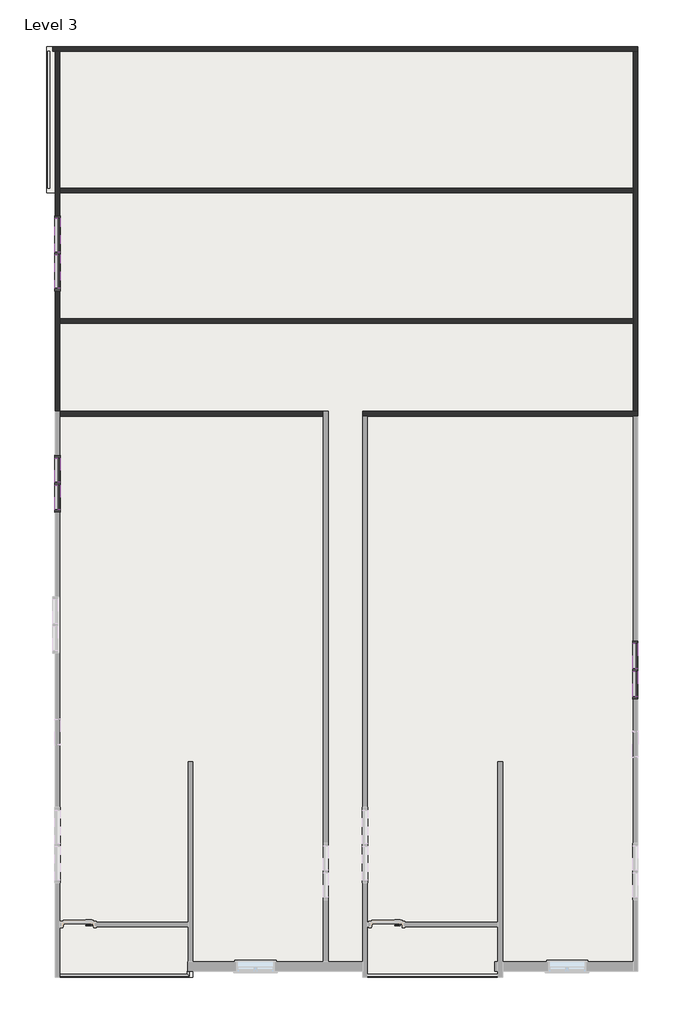
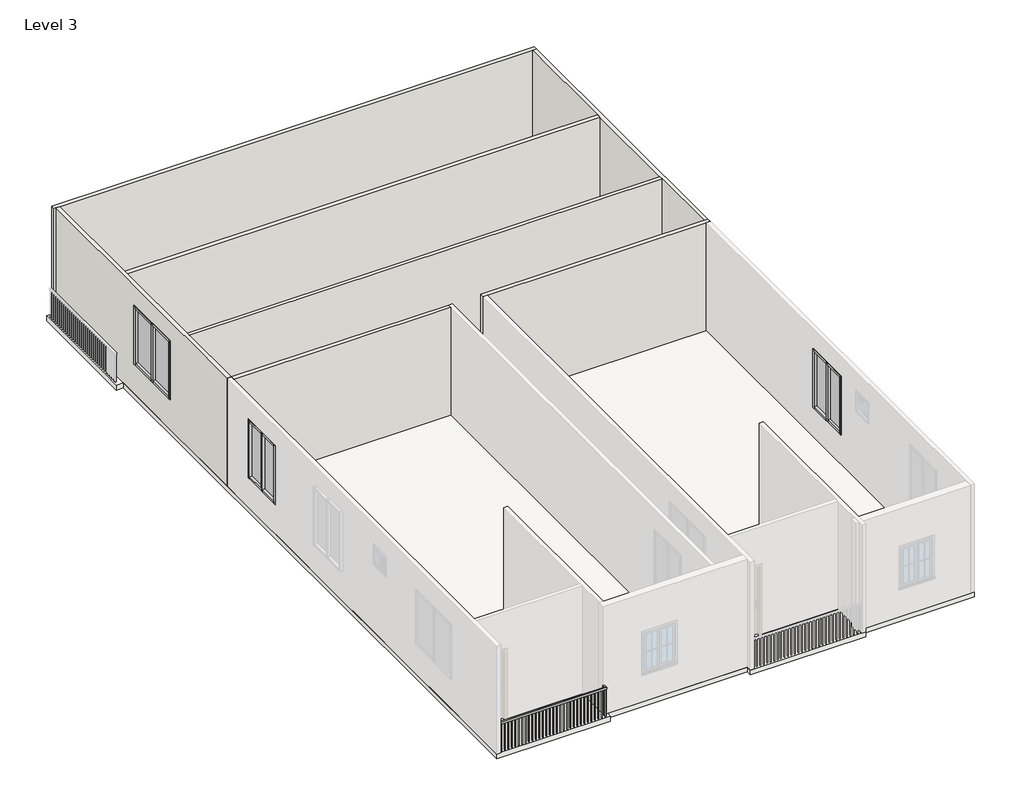
# One storey, part 2 of 3: 21 members, 7 walls, 6 plates, 1 railing, 1 slab.
"""IFC4 building model written with IfcOpenShell, lengths in millimetres."""

from ifc_helpers import new_model, si_unit, frame, origin, place, context, project, spatial, polyline, outline, extrude, faceted_brep, transform, mapped, element, save
from components import member_3f0e0172, member_96ae0c19, member_d60e8053, member_2fae0574, member_3e1d4a65, system_panel_glazed_c4393626, system_panel_glazed_d2c73f4b, system_panel_glazed_30879ba3

model = new_model("IFC4")

# Units and contexts
model_context = context("Model", 3, world=origin())
ifc_project = project(units=[si_unit("LENGTHUNIT", "METRE", prefix="MILLI")], contexts=[model_context])

# Site, building, storey
site = spatial("IfcSite", under=ifc_project)
building = spatial("IfcBuilding", under=site)
storey = spatial("IfcBuildingStorey", under=building, Name="Level 3", Elevation=6705.6)

# Members
placement = place(None, origin())
member_shape = member_3f0e0172(model_context)
element("IfcMember", 1, ObjectType="Rectangular Mullion : 2.5\" x 5\" rectangular", at=placement, inside=storey, context=model_context, shape_type="MappedRepresentation", body=[
    mapped(member_shape, transform((5848.1708786, -3933.7021821, 9448.8), x_axis=(0.0, 0.0, 1.0), y_axis=(-1.0, 0.0, 0.0), z_axis=(0.0, -1.0, 0.0))),
])
element("IfcMember", 2, ObjectType="Rectangular Mullion : 2.5\" x 5\" rectangular", at=placement, inside=storey, context=model_context, shape_type="MappedRepresentation", body=[
    mapped(member_shape, transform((5848.1708786, -3254.2521821, 9448.8), x_axis=(0.0, 0.0, 1.0), y_axis=(-1.0, 0.0, 0.0), z_axis=(0.0, -1.0, 0.0))),
])
element("IfcMember", 3, ObjectType="Rectangular Mullion : 2.5\" x 5\" rectangular", at=placement, inside=storey, context=model_context, shape_type="MappedRepresentation", body=[
    mapped(member_shape, transform((5848.1708786, -2638.3021821, 7620.0), x_axis=(0.0, 0.0, -1.0), y_axis=(-1.0, 0.0, 0.0), z_axis=(0.0, 1.0, 0.0))),
])
element("IfcMember", 4, ObjectType="Rectangular Mullion : 2.5\" x 5\" rectangular", at=placement, inside=storey, context=model_context, shape_type="MappedRepresentation", body=[
    mapped(member_shape, transform((5848.1708786, -3317.7521821, 7620.0), x_axis=(0.0, 0.0, -1.0), y_axis=(-1.0, 0.0, 0.0), z_axis=(0.0, 1.0, 0.0))),
])
member_2_shape = member_96ae0c19(model_context)
element("IfcMember", 5, ObjectType="Rectangular Mullion : 2.5\" x 5\" rectangular", at=placement, inside=storey, context=model_context, shape_type="MappedRepresentation", body=[
    mapped(member_2_shape, transform((-8153.157583, 600.1666267, 9448.8), x_axis=(0.0, 0.0, 1.0), y_axis=(-1.0, 0.0, 0.0), z_axis=(0.0, -1.0, 0.0))),
])
element("IfcMember", 6, ObjectType="Rectangular Mullion : 2.5\" x 5\" rectangular", at=placement, inside=storey, context=model_context, shape_type="MappedRepresentation", body=[
    mapped(member_2_shape, transform((-8153.157583, 1254.9937905, 9448.8), x_axis=(0.0, 0.0, 1.0), y_axis=(-1.0, 0.0, 0.0), z_axis=(0.0, -1.0, 0.0))),
])
element("IfcMember", 7, ObjectType="Rectangular Mullion : 2.5\" x 5\" rectangular", at=placement, inside=storey, context=model_context, shape_type="MappedRepresentation", body=[
    mapped(member_2_shape, transform((-8153.157583, 1846.3209543, 7620.0), x_axis=(0.0, 0.0, -1.0), y_axis=(-1.0, 0.0, 0.0), z_axis=(0.0, 1.0, 0.0))),
])
element("IfcMember", 8, ObjectType="Rectangular Mullion : 2.5\" x 5\" rectangular", at=placement, inside=storey, context=model_context, shape_type="MappedRepresentation", body=[
    mapped(member_2_shape, transform((-8153.157583, 1191.4937905, 7620.0), x_axis=(0.0, 0.0, -1.0), y_axis=(-1.0, 0.0, 0.0), z_axis=(0.0, 1.0, 0.0))),
])
member_3_shape = member_d60e8053(model_context)
element("IfcMember", 9, ObjectType="Rectangular Mullion : 2.5\" x 5\" rectangular", at=placement, inside=storey, context=model_context, shape_type="MappedRepresentation", body=[
    mapped(member_3_shape, transform((5848.1708786, -3286.0021821, 7620.0), x_axis=(0.0, -1.0, 0.0), y_axis=(-1.0, 0.0, 0.0), z_axis=(0.0, 0.0, -1.0))),
])
element("IfcMember", 10, ObjectType="Rectangular Mullion : 2.5\" x 5\" rectangular", at=placement, inside=storey, context=model_context, shape_type="MappedRepresentation", body=[
    mapped(member_3_shape, transform((-8153.157583, 1223.2437905, 7620.0), x_axis=(0.0, -1.0, 0.0), y_axis=(-1.0, 0.0, 0.0), z_axis=(0.0, 0.0, -1.0))),
])
element("IfcMember", 11, ObjectType="Rectangular Mullion : 2.5\" x 5\" rectangular", at=placement, inside=storey, context=model_context, shape_type="MappedRepresentation", body=[
    mapped(member_3_shape, transform((-8153.157583, 6807.1511393, 7620.0), x_axis=(0.0, -1.0, 0.0), y_axis=(-1.0, 0.0, 0.0), z_axis=(0.0, 0.0, -1.0))),
])
member_4_shape = member_2fae0574(model_context)
element("IfcMember", 12, ObjectType="Rectangular Mullion : 2.5\" x 5\" rectangular", at=placement, inside=storey, context=model_context, shape_type="MappedRepresentation", body=[
    mapped(member_4_shape, transform((5848.1708786, -2574.8021821, 9448.8), x_axis=(0.0, 1.0, 0.0), y_axis=(-1.0, 0.0, 0.0), z_axis=(0.0, 0.0, 1.0))),
])
element("IfcMember", 13, ObjectType="Rectangular Mullion : 2.5\" x 5\" rectangular", at=placement, inside=storey, context=model_context, shape_type="MappedRepresentation", body=[
    mapped(member_4_shape, transform((-8153.157583, 1909.8209543, 9448.8), x_axis=(0.0, 1.0, 0.0), y_axis=(-1.0, 0.0, 0.0), z_axis=(0.0, 0.0, 1.0))),
])
element("IfcMember", 14, ObjectType="Rectangular Mullion : 2.5\" x 5\" rectangular", at=placement, inside=storey, context=model_context, shape_type="MappedRepresentation", body=[
    mapped(member_4_shape, transform((-8153.157583, 7721.9533991, 9448.8), x_axis=(0.0, 1.0, 0.0), y_axis=(-1.0, 0.0, 0.0), z_axis=(0.0, 0.0, 1.0))),
])
element("IfcMember", 15, ObjectType="Rectangular Mullion : 2.5\" x 5\" rectangular", at=placement, inside=storey, context=model_context, shape_type="MappedRepresentation", body=[
    mapped(member_4_shape, transform((5848.1708786, -3997.2021821, 7620.0), x_axis=(0.0, -1.0, 0.0), y_axis=(-1.0, 0.0, 0.0), z_axis=(0.0, 0.0, -1.0))),
])
element("IfcMember", 16, ObjectType="Rectangular Mullion : 2.5\" x 5\" rectangular", at=placement, inside=storey, context=model_context, shape_type="MappedRepresentation", body=[
    mapped(member_4_shape, transform((-8153.157583, 536.6666267, 7620.0), x_axis=(0.0, -1.0, 0.0), y_axis=(-1.0, 0.0, 0.0), z_axis=(0.0, 0.0, -1.0))),
])
element("IfcMember", 17, ObjectType="Rectangular Mullion : 2.5\" x 5\" rectangular", at=placement, inside=storey, context=model_context, shape_type="MappedRepresentation", body=[
    mapped(member_4_shape, transform((-8153.157583, 5892.3488795, 7620.0), x_axis=(0.0, -1.0, 0.0), y_axis=(-1.0, 0.0, 0.0), z_axis=(0.0, 0.0, -1.0))),
])
member_5_shape = member_3e1d4a65(model_context)
element("IfcMember", 18, ObjectType="Rectangular Mullion : 2.5\" x 5\" rectangular", at=placement, inside=storey, context=model_context, shape_type="MappedRepresentation", body=[
    mapped(member_5_shape, transform((-8153.157583, 5955.8488795, 9448.8), x_axis=(0.0, 0.0, 1.0), y_axis=(-1.0, 0.0, 0.0), z_axis=(0.0, -1.0, 0.0))),
])
element("IfcMember", 19, ObjectType="Rectangular Mullion : 2.5\" x 5\" rectangular", at=placement, inside=storey, context=model_context, shape_type="MappedRepresentation", body=[
    mapped(member_5_shape, transform((-8153.157583, 6838.9011393, 9448.8), x_axis=(0.0, 0.0, 1.0), y_axis=(-1.0, 0.0, 0.0), z_axis=(0.0, -1.0, 0.0))),
])
element("IfcMember", 20, ObjectType="Rectangular Mullion : 2.5\" x 5\" rectangular", at=placement, inside=storey, context=model_context, shape_type="MappedRepresentation", body=[
    mapped(member_5_shape, transform((-8153.157583, 7658.4533991, 7620.0), x_axis=(0.0, 0.0, -1.0), y_axis=(-1.0, 0.0, 0.0), z_axis=(0.0, 1.0, 0.0))),
])
element("IfcMember", 21, ObjectType="Rectangular Mullion : 2.5\" x 5\" rectangular", at=placement, inside=storey, context=model_context, shape_type="MappedRepresentation", body=[
    mapped(member_5_shape, transform((-8153.157583, 6775.4011393, 7620.0), x_axis=(0.0, 0.0, -1.0), y_axis=(-1.0, 0.0, 0.0), z_axis=(0.0, 1.0, 0.0))),
])

# Plates
system_panel_glazed_shape = system_panel_glazed_c4393626(model_context)
element("IfcPlate", 22, ObjectType="System Panel : Glazed", at=placement, inside=storey, context=model_context, shape_type="MappedRepresentation", body=[
    mapped(system_panel_glazed_shape, transform((-8153.157583, 1550.6573724, 7683.5), x_axis=(0.0, -1.0, 0.0), y_axis=(1.0, 0.0, 0.0), z_axis=(0.0, 0.0, 1.0))),
])
element("IfcPlate", 23, ObjectType="System Panel : Glazed", at=placement, inside=storey, context=model_context, shape_type="MappedRepresentation", body=[
    mapped(system_panel_glazed_shape, transform((-8153.157583, 895.8302086, 7683.5), x_axis=(0.0, -1.0, 0.0), y_axis=(1.0, 0.0, 0.0), z_axis=(0.0, 0.0, 1.0))),
])
system_panel_glazed_2_shape = system_panel_glazed_d2c73f4b(model_context)
element("IfcPlate", 24, ObjectType="System Panel : Glazed", at=placement, inside=storey, context=model_context, shape_type="MappedRepresentation", body=[
    mapped(system_panel_glazed_2_shape, transform((5848.1708786, -2946.2771821, 7683.5), x_axis=(0.0, -1.0, 0.0), y_axis=(1.0, 0.0, 0.0), z_axis=(0.0, 0.0, 1.0))),
])
element("IfcPlate", 25, ObjectType="System Panel : Glazed", at=placement, inside=storey, context=model_context, shape_type="MappedRepresentation", body=[
    mapped(system_panel_glazed_2_shape, transform((5848.1708786, -3625.7271821, 7683.5), x_axis=(0.0, -1.0, 0.0), y_axis=(1.0, 0.0, 0.0), z_axis=(0.0, 0.0, 1.0))),
])
system_panel_glazed_3_shape = system_panel_glazed_30879ba3(model_context)
element("IfcPlate", 26, ObjectType="System Panel : Glazed", at=placement, inside=storey, context=model_context, shape_type="MappedRepresentation", body=[
    mapped(system_panel_glazed_3_shape, transform((-8153.157583, 7248.6772692, 7683.5), x_axis=(0.0, -1.0, 0.0), y_axis=(1.0, 0.0, 0.0), z_axis=(0.0, 0.0, 1.0))),
])
element("IfcPlate", 27, ObjectType="System Panel : Glazed", at=placement, inside=storey, context=model_context, shape_type="MappedRepresentation", body=[
    mapped(system_panel_glazed_3_shape, transform((-8153.157583, 6365.6250094, 7683.5), x_axis=(0.0, -1.0, 0.0), y_axis=(1.0, 0.0, 0.0), z_axis=(0.0, 0.0, 1.0))),
])

# Railing
element("IfcRailing", 28, ObjectType="Handrail - Rectangular", at=placement, inside=storey, context=model_context, shape_type="SolidModel", body=[
    faceted_brep([(-8153.157583, -10659.0005933, 7620.0), (-8153.157583, -10659.0005933, 7569.2), (-8153.157583, -10709.8005933, 7569.2), (-8153.157583, -10709.8005933, 7620.0), (-5014.0237038, -10659.0005933, 7620.0), (-5014.0237038, -10659.0005933, 7569.2), (-4963.2237038, -10709.8005933, 7569.2), (-4963.2237038, -10709.8005933, 7620.0), (-5014.0237038, -10582.0742041, 7620.0), (-4963.2237038, -10582.0742041, 7620.0), (-4963.2237038, -10582.0742041, 7569.2), (-5014.0237038, -10582.0742041, 7569.2)], [[[0, 1, 2, 3]], [[1, 0, 4, 5]], [[2, 1, 5, 6]], [[3, 2, 6, 7]], [[0, 3, 7, 4]], [[8, 9, 10, 11]], [[5, 4, 8, 11]], [[6, 5, 11, 10]], [[7, 6, 10, 9]], [[4, 7, 9, 8]]]),
    extrude(outline(polyline([(-4979.0987038, -10592.3255933), (-4998.1487038, -10592.3255933), (-4998.1487038, -10573.2755933), (-4979.0987038, -10573.2755933), (-4979.0987038, -10592.3255933)])), frame((0.0, 0.0, 6705.6), z_axis=(0.0, 0.0, 1.0), x_axis=(1.0, 0.0, 0.0)), (0.0, 0.0, 1.0), 863.6),
    extrude(outline(polyline([(-5013.082583, -10693.9255933), (-5013.082583, -10674.8755933), (-4994.032583, -10674.8755933), (-4994.032583, -10693.9255933), (-5013.082583, -10693.9255933)])), frame((0.0, 0.0, 6705.6), z_axis=(0.0, 0.0, 1.0), x_axis=(1.0, 0.0, 0.0)), (0.0, 0.0, 1.0), 863.6),
    extrude(outline(polyline([(-5114.682583, -10693.9255933), (-5114.682583, -10674.8755933), (-5095.632583, -10674.8755933), (-5095.632583, -10693.9255933), (-5114.682583, -10693.9255933)])), frame((0.0, 0.0, 6705.6), z_axis=(0.0, 0.0, 1.0), x_axis=(1.0, 0.0, 0.0)), (0.0, 0.0, 1.0), 863.6),
    extrude(outline(polyline([(-5216.282583, -10693.9255933), (-5216.282583, -10674.8755933), (-5197.232583, -10674.8755933), (-5197.232583, -10693.9255933), (-5216.282583, -10693.9255933)])), frame((0.0, 0.0, 6705.6), z_axis=(0.0, 0.0, 1.0), x_axis=(1.0, 0.0, 0.0)), (0.0, 0.0, 1.0), 863.6),
    extrude(outline(polyline([(-5317.882583, -10693.9255933), (-5317.882583, -10674.8755933), (-5298.832583, -10674.8755933), (-5298.832583, -10693.9255933), (-5317.882583, -10693.9255933)])), frame((0.0, 0.0, 6705.6), z_axis=(0.0, 0.0, 1.0), x_axis=(1.0, 0.0, 0.0)), (0.0, 0.0, 1.0), 863.6),
    extrude(outline(polyline([(-5419.482583, -10693.9255933), (-5419.482583, -10674.8755933), (-5400.432583, -10674.8755933), (-5400.432583, -10693.9255933), (-5419.482583, -10693.9255933)])), frame((0.0, 0.0, 6705.6), z_axis=(0.0, 0.0, 1.0), x_axis=(1.0, 0.0, 0.0)), (0.0, 0.0, 1.0), 863.6),
    extrude(outline(polyline([(-5521.082583, -10693.9255933), (-5521.082583, -10674.8755933), (-5502.032583, -10674.8755933), (-5502.032583, -10693.9255933), (-5521.082583, -10693.9255933)])), frame((0.0, 0.0, 6705.6), z_axis=(0.0, 0.0, 1.0), x_axis=(1.0, 0.0, 0.0)), (0.0, 0.0, 1.0), 863.6),
    extrude(outline(polyline([(-5622.682583, -10693.9255933), (-5622.682583, -10674.8755933), (-5603.632583, -10674.8755933), (-5603.632583, -10693.9255933), (-5622.682583, -10693.9255933)])), frame((0.0, 0.0, 6705.6), z_axis=(0.0, 0.0, 1.0), x_axis=(1.0, 0.0, 0.0)), (0.0, 0.0, 1.0), 863.6),
    extrude(outline(polyline([(-5724.282583, -10693.9255933), (-5724.282583, -10674.8755933), (-5705.232583, -10674.8755933), (-5705.232583, -10693.9255933), (-5724.282583, -10693.9255933)])), frame((0.0, 0.0, 6705.6), z_axis=(0.0, 0.0, 1.0), x_axis=(1.0, 0.0, 0.0)), (0.0, 0.0, 1.0), 863.6),
    extrude(outline(polyline([(-5825.882583, -10693.9255933), (-5825.882583, -10674.8755933), (-5806.832583, -10674.8755933), (-5806.832583, -10693.9255933), (-5825.882583, -10693.9255933)])), frame((0.0, 0.0, 6705.6), z_axis=(0.0, 0.0, 1.0), x_axis=(1.0, 0.0, 0.0)), (0.0, 0.0, 1.0), 863.6),
    extrude(outline(polyline([(-5927.482583, -10693.9255933), (-5927.482583, -10674.8755933), (-5908.432583, -10674.8755933), (-5908.432583, -10693.9255933), (-5927.482583, -10693.9255933)])), frame((0.0, 0.0, 6705.6), z_axis=(0.0, 0.0, 1.0), x_axis=(1.0, 0.0, 0.0)), (0.0, 0.0, 1.0), 863.6),
    extrude(outline(polyline([(-6029.082583, -10693.9255933), (-6029.082583, -10674.8755933), (-6010.032583, -10674.8755933), (-6010.032583, -10693.9255933), (-6029.082583, -10693.9255933)])), frame((0.0, 0.0, 6705.6), z_axis=(0.0, 0.0, 1.0), x_axis=(1.0, 0.0, 0.0)), (0.0, 0.0, 1.0), 863.6),
    extrude(outline(polyline([(-6130.682583, -10693.9255933), (-6130.682583, -10674.8755933), (-6111.632583, -10674.8755933), (-6111.632583, -10693.9255933), (-6130.682583, -10693.9255933)])), frame((0.0, 0.0, 6705.6), z_axis=(0.0, 0.0, 1.0), x_axis=(1.0, 0.0, 0.0)), (0.0, 0.0, 1.0), 863.6),
    extrude(outline(polyline([(-6232.282583, -10693.9255933), (-6232.282583, -10674.8755933), (-6213.232583, -10674.8755933), (-6213.232583, -10693.9255933), (-6232.282583, -10693.9255933)])), frame((0.0, 0.0, 6705.6), z_axis=(0.0, 0.0, 1.0), x_axis=(1.0, 0.0, 0.0)), (0.0, 0.0, 1.0), 863.6),
    extrude(outline(polyline([(-6333.882583, -10693.9255933), (-6333.882583, -10674.8755933), (-6314.832583, -10674.8755933), (-6314.832583, -10693.9255933), (-6333.882583, -10693.9255933)])), frame((0.0, 0.0, 6705.6), z_axis=(0.0, 0.0, 1.0), x_axis=(1.0, 0.0, 0.0)), (0.0, 0.0, 1.0), 863.6),
    extrude(outline(polyline([(-6435.482583, -10693.9255933), (-6435.482583, -10674.8755933), (-6416.432583, -10674.8755933), (-6416.432583, -10693.9255933), (-6435.482583, -10693.9255933)])), frame((0.0, 0.0, 6705.6), z_axis=(0.0, 0.0, 1.0), x_axis=(1.0, 0.0, 0.0)), (0.0, 0.0, 1.0), 863.6),
    extrude(outline(polyline([(-6537.082583, -10693.9255933), (-6537.082583, -10674.8755933), (-6518.032583, -10674.8755933), (-6518.032583, -10693.9255933), (-6537.082583, -10693.9255933)])), frame((0.0, 0.0, 6705.6), z_axis=(0.0, 0.0, 1.0), x_axis=(1.0, 0.0, 0.0)), (0.0, 0.0, 1.0), 863.6),
    extrude(outline(polyline([(-6638.682583, -10693.9255933), (-6638.682583, -10674.8755933), (-6619.632583, -10674.8755933), (-6619.632583, -10693.9255933), (-6638.682583, -10693.9255933)])), frame((0.0, 0.0, 6705.6), z_axis=(0.0, 0.0, 1.0), x_axis=(1.0, 0.0, 0.0)), (0.0, 0.0, 1.0), 863.6),
    extrude(outline(polyline([(-6740.282583, -10693.9255933), (-6740.282583, -10674.8755933), (-6721.232583, -10674.8755933), (-6721.232583, -10693.9255933), (-6740.282583, -10693.9255933)])), frame((0.0, 0.0, 6705.6), z_axis=(0.0, 0.0, 1.0), x_axis=(1.0, 0.0, 0.0)), (0.0, 0.0, 1.0), 863.6),
    extrude(outline(polyline([(-6841.882583, -10693.9255933), (-6841.882583, -10674.8755933), (-6822.832583, -10674.8755933), (-6822.832583, -10693.9255933), (-6841.882583, -10693.9255933)])), frame((0.0, 0.0, 6705.6), z_axis=(0.0, 0.0, 1.0), x_axis=(1.0, 0.0, 0.0)), (0.0, 0.0, 1.0), 863.6),
    extrude(outline(polyline([(-6943.482583, -10693.9255933), (-6943.482583, -10674.8755933), (-6924.432583, -10674.8755933), (-6924.432583, -10693.9255933), (-6943.482583, -10693.9255933)])), frame((0.0, 0.0, 6705.6), z_axis=(0.0, 0.0, 1.0), x_axis=(1.0, 0.0, 0.0)), (0.0, 0.0, 1.0), 863.6),
    extrude(outline(polyline([(-7045.082583, -10693.9255933), (-7045.082583, -10674.8755933), (-7026.032583, -10674.8755933), (-7026.032583, -10693.9255933), (-7045.082583, -10693.9255933)])), frame((0.0, 0.0, 6705.6), z_axis=(0.0, 0.0, 1.0), x_axis=(1.0, 0.0, 0.0)), (0.0, 0.0, 1.0), 863.6),
    extrude(outline(polyline([(-7146.682583, -10693.9255933), (-7146.682583, -10674.8755933), (-7127.632583, -10674.8755933), (-7127.632583, -10693.9255933), (-7146.682583, -10693.9255933)])), frame((0.0, 0.0, 6705.6), z_axis=(0.0, 0.0, 1.0), x_axis=(1.0, 0.0, 0.0)), (0.0, 0.0, 1.0), 863.6),
    extrude(outline(polyline([(-7248.282583, -10693.9255933), (-7248.282583, -10674.8755933), (-7229.232583, -10674.8755933), (-7229.232583, -10693.9255933), (-7248.282583, -10693.9255933)])), frame((0.0, 0.0, 6705.6), z_axis=(0.0, 0.0, 1.0), x_axis=(1.0, 0.0, 0.0)), (0.0, 0.0, 1.0), 863.6),
    extrude(outline(polyline([(-7349.882583, -10693.9255933), (-7349.882583, -10674.8755933), (-7330.832583, -10674.8755933), (-7330.832583, -10693.9255933), (-7349.882583, -10693.9255933)])), frame((0.0, 0.0, 6705.6), z_axis=(0.0, 0.0, 1.0), x_axis=(1.0, 0.0, 0.0)), (0.0, 0.0, 1.0), 863.6),
    extrude(outline(polyline([(-7451.482583, -10693.9255933), (-7451.482583, -10674.8755933), (-7432.432583, -10674.8755933), (-7432.432583, -10693.9255933), (-7451.482583, -10693.9255933)])), frame((0.0, 0.0, 6705.6), z_axis=(0.0, 0.0, 1.0), x_axis=(1.0, 0.0, 0.0)), (0.0, 0.0, 1.0), 863.6),
    extrude(outline(polyline([(-7553.082583, -10693.9255933), (-7553.082583, -10674.8755933), (-7534.032583, -10674.8755933), (-7534.032583, -10693.9255933), (-7553.082583, -10693.9255933)])), frame((0.0, 0.0, 6705.6), z_axis=(0.0, 0.0, 1.0), x_axis=(1.0, 0.0, 0.0)), (0.0, 0.0, 1.0), 863.6),
    extrude(outline(polyline([(-7654.682583, -10693.9255933), (-7654.682583, -10674.8755933), (-7635.632583, -10674.8755933), (-7635.632583, -10693.9255933), (-7654.682583, -10693.9255933)])), frame((0.0, 0.0, 6705.6), z_axis=(0.0, 0.0, 1.0), x_axis=(1.0, 0.0, 0.0)), (0.0, 0.0, 1.0), 863.6),
    extrude(outline(polyline([(-7756.282583, -10693.9255933), (-7756.282583, -10674.8755933), (-7737.232583, -10674.8755933), (-7737.232583, -10693.9255933), (-7756.282583, -10693.9255933)])), frame((0.0, 0.0, 6705.6), z_axis=(0.0, 0.0, 1.0), x_axis=(1.0, 0.0, 0.0)), (0.0, 0.0, 1.0), 863.6),
    extrude(outline(polyline([(-7857.882583, -10693.9255933), (-7857.882583, -10674.8755933), (-7838.832583, -10674.8755933), (-7838.832583, -10693.9255933), (-7857.882583, -10693.9255933)])), frame((0.0, 0.0, 6705.6), z_axis=(0.0, 0.0, 1.0), x_axis=(1.0, 0.0, 0.0)), (0.0, 0.0, 1.0), 863.6),
    extrude(outline(polyline([(-7959.482583, -10693.9255933), (-7959.482583, -10674.8755933), (-7940.432583, -10674.8755933), (-7940.432583, -10693.9255933), (-7959.482583, -10693.9255933)])), frame((0.0, 0.0, 6705.6), z_axis=(0.0, 0.0, 1.0), x_axis=(1.0, 0.0, 0.0)), (0.0, 0.0, 1.0), 863.6),
    extrude(outline(polyline([(-8061.082583, -10693.9255933), (-8061.082583, -10674.8755933), (-8042.032583, -10674.8755933), (-8042.032583, -10693.9255933), (-8061.082583, -10693.9255933)])), frame((0.0, 0.0, 6705.6), z_axis=(0.0, 0.0, 1.0), x_axis=(1.0, 0.0, 0.0)), (0.0, 0.0, 1.0), 863.6),
    extrude(outline(polyline([(-4998.1487038, -10693.9255933), (-4998.1487038, -10674.8755933), (-4979.0987038, -10674.8755933), (-4979.0987038, -10693.9255933), (-4998.1487038, -10693.9255933)])), frame((0.0, 0.0, 6705.6), z_axis=(0.0, 0.0, 1.0), x_axis=(1.0, 0.0, 0.0)), (0.0, 0.0, 1.0), 863.6),
    extrude(outline(polyline([(-4979.0987038, -10601.1242041), (-4998.1487038, -10601.1242041), (-4998.1487038, -10582.0742041), (-4979.0987038, -10582.0742041), (-4979.0987038, -10601.1242041)])), frame((0.0, 0.0, 6705.6), z_axis=(0.0, 0.0, 1.0), x_axis=(1.0, 0.0, 0.0)), (0.0, 0.0, 1.0), 863.6),
    extrude(outline(polyline([(-8153.157583, -10693.9255933), (-8153.157583, -10674.8755933), (-8134.107583, -10674.8755933), (-8134.107583, -10693.9255933), (-8153.157583, -10693.9255933)])), frame((0.0, 0.0, 6705.6), z_axis=(0.0, 0.0, 1.0), x_axis=(1.0, 0.0, 0.0)), (0.0, 0.0, 1.0), 863.6),
])

# Slab
element("IfcSlab", 29, ObjectType="6\" floor", at=placement, inside=storey, context=model_context, shape_type="SweptSolid", body=[
    extrude(outline(polyline([(5905.3208786, 11818.2189683), (5905.3208786, -10585.8779557), (2630.290751, -10585.8779557), (2630.290751, -10737.6531157), (-762.8431282, -10737.6531157), (-762.8431282, -10585.8779557), (-4874.3237038, -10585.8779557), (-4874.3237038, -10733.8493641), (-8210.307583, -10733.8493641), (-8210.307583, 8277.3011327), (-8419.607647, 8277.3011327), (-8419.607647, 11818.2189683), (5905.3208786, 11818.2189683)])), frame((0.0, 0.0, 6553.2), z_axis=(0.0, 0.0, 1.0), x_axis=(1.0, 0.0, 0.0)), (0.0, 0.0, 1.0), 152.4),
])

# Walls
element("IfcWall", 30, ObjectType="4.5\" wall", at=placement, inside=storey, context=model_context, shape_type="Brep", body=[
    faceted_brep([(-8267.457583, 11703.9189683, 6705.6), (-8210.307583, 11703.9189683, 6705.6), (-8096.007583, 11703.9189683, 6705.6), (5791.0208786, 11703.9189683, 6705.6), (5905.3208786, 11703.9189683, 6705.6), (5905.3208786, 11703.9189683, 10058.4), (5791.0208786, 11703.9189683, 10058.4), (-8096.007583, 11703.9189683, 10058.4), (-8210.307583, 11703.9189683, 10058.4), (-8267.457583, 11703.9189683, 10058.4), (-8267.457583, 11818.2189683, 6705.6), (-8267.457583, 11818.2189683, 10058.4), (5905.3208786, 11818.2189683, 10058.4), (5905.3208786, 11818.2189683, 6705.6)], [[[0, 1, 2, 3, 4, 5, 6, 7, 8, 9]], [[10, 11, 12, 13]], [[4, 3, 2, 1, 0, 10, 13]], [[9, 8, 7, 6, 5, 12, 11]], [[0, 9, 11, 10]], [[5, 4, 13, 12]]]),
])
element("IfcWall", 31, ObjectType="4.5\" wall", at=placement, inside=storey, context=model_context, shape_type="Brep", body=[
    faceted_brep([(5791.0208786, 11703.9189683, 6705.6), (5791.0208786, 8387.4224771, 6705.6), (5791.0208786, 8273.1224771, 6705.6), (5791.0208786, 5226.5048975, 6705.6), (5791.0208786, 5112.2048975, 6705.6), (5791.0208786, 2978.3002499, 6705.6), (5791.0208786, 2978.3002499, 10058.4), (5791.0208786, 5112.2048975, 10058.4), (5791.0208786, 5226.5048975, 10058.4), (5791.0208786, 8273.1224771, 10058.4), (5791.0208786, 8387.4224771, 10058.4), (5791.0208786, 11703.9189683, 10058.4), (5905.3208786, 11703.9189683, 6705.6), (5905.3208786, 11703.9189683, 10058.4), (5905.3208786, 2978.3002499, 10058.4), (5905.3208786, 2978.3002499, 6705.6)], [[[0, 1, 2, 3, 4, 5, 6, 7, 8, 9, 10, 11]], [[12, 13, 14, 15]], [[5, 4, 3, 2, 1, 0, 12, 15]], [[11, 10, 9, 8, 7, 6, 14, 13]], [[0, 11, 13, 12]], [[6, 5, 15, 14]]]),
])
element("IfcWall", 32, ObjectType="4.5\" wall", at=placement, inside=storey, context=model_context, shape_type="SweptSolid", body=[
    extrude(outline(polyline([(-1713.5935762, 2864.0002499), (-8096.007583, 2864.0002499), (-8096.007583, 2978.3002499), (-1713.5935762, 2978.3002499), (-1713.5935762, 2864.0002499)])), frame((0.0, 0.0, 6705.6), z_axis=(0.0, 0.0, 1.0), x_axis=(1.0, 0.0, 0.0)), (0.0, 0.0, 1.0), 3352.8),
])
element("IfcWall", 33, ObjectType="4.5\" wall", at=placement, inside=storey, context=model_context, shape_type="SweptSolid", body=[
    extrude(outline(polyline([(-8096.007583, 5226.5048975), (5791.0208786, 5226.5048975), (5791.0208786, 5112.2048975), (-8096.007583, 5112.2048975), (-8096.007583, 5226.5048975)])), frame((0.0, 0.0, 6705.6), z_axis=(0.0, 0.0, 1.0), x_axis=(1.0, 0.0, 0.0)), (0.0, 0.0, 1.0), 3352.8),
])
element("IfcWall", 34, ObjectType="4.5\" wall", at=placement, inside=storey, context=model_context, shape_type="SweptSolid", body=[
    extrude(outline(polyline([(-8096.007583, 8387.4224771), (5791.0208786, 8387.4224771), (5791.0208786, 8273.1224771), (-8096.007583, 8273.1224771), (-8096.007583, 8387.4224771)])), frame((0.0, 0.0, 6705.6), z_axis=(0.0, 0.0, 1.0), x_axis=(1.0, 0.0, 0.0)), (0.0, 0.0, 1.0), 3352.8),
])
element("IfcWall", 35, ObjectType="4.5\" wall", at=placement, inside=storey, context=model_context, shape_type="Brep", body=[
    faceted_brep([(-8096.007583, 2978.3002499, 6705.6), (-8096.007583, 5112.2048975, 6705.6), (-8096.007583, 5226.5048975, 6705.6), (-8096.007583, 8273.1224771, 6705.6), (-8096.007583, 8387.4224771, 6705.6), (-8096.007583, 11703.9189683, 6705.6), (-8096.007583, 11703.9189683, 10058.4), (-8096.007583, 8387.4224771, 10058.4), (-8096.007583, 8273.1224771, 10058.4), (-8096.007583, 5226.5048975, 10058.4), (-8096.007583, 5112.2048975, 10058.4), (-8096.007583, 2978.3002499, 10058.4), (-8096.007583, 7721.9533991, 9448.8), (-8096.007583, 7721.9533991, 7620.0), (-8096.007583, 5892.3488795, 7620.0), (-8096.007583, 5892.3488795, 9448.8), (-8210.307583, 11703.9189683, 6705.6), (-8210.307583, 2978.3002499, 6705.6), (-8210.307583, 2978.3002499, 10058.4), (-8210.307583, 11703.9189683, 10058.4), (-8210.307583, 7721.9533991, 7620.0), (-8210.307583, 7721.9533991, 9448.8), (-8210.307583, 5892.3488795, 9448.8), (-8210.307583, 5892.3488795, 7620.0)], [[[0, 1, 2, 3, 4, 5, 6, 7, 8, 9, 10, 11], [12, 13, 14, 15]], [[16, 17, 18, 19], [20, 21, 22, 23]], [[5, 4, 3, 2, 1, 0, 17, 16]], [[11, 10, 9, 8, 7, 6, 19, 18]], [[6, 5, 16, 19]], [[0, 11, 18, 17]], [[20, 13, 12, 21]], [[21, 12, 15, 22]], [[22, 15, 14, 23]], [[13, 20, 23, 14]]]),
])
element("IfcWall", 36, ObjectType="4.5\" wall", at=placement, inside=storey, context=model_context, shape_type="Brep", body=[
    faceted_brep([(-762.8431282, 2864.0002499, 6705.6), (-648.5431282, 2864.0002499, 6705.6), (5791.0208786, 2864.0002499, 6705.6), (5905.3208786, 2864.0002499, 6705.6), (5905.3208786, 2864.0002499, 10058.4), (5791.0208786, 2864.0002499, 10058.4), (-648.5431282, 2864.0002499, 10058.4), (-762.8431282, 2864.0002499, 10058.4), (-762.8431282, 2978.3002499, 6705.6), (-762.8431282, 2978.3002499, 10058.4), (5791.0208786, 2978.3002499, 10058.4), (5905.3208786, 2978.3002499, 10058.4), (5905.3208786, 2978.3002499, 6705.6), (5791.0208786, 2978.3002499, 6705.6)], [[[0, 1, 2, 3, 4, 5, 6, 7]], [[8, 9, 10, 11, 12, 13]], [[3, 2, 1, 0, 8, 13, 12]], [[7, 6, 5, 4, 11, 10, 9]], [[4, 3, 12, 11]], [[0, 7, 9, 8]]]),
])

save(model, "model.ifc")

# Revit data of these elements
# Type "Rectangular Mullion : 2.5\" x 5\" rectangular"
#   built-in parameter 1007304 = 0.416667 (stored number, unit not read)
#   built-in parameter 1007301 = 0.104167 (stored number, unit not read)
#   built-in parameter 1007300 = 0.104167 (stored number, unit not read)
# Type "System Panel : Glazed"
#   Construction Type Id = "GSP4R"
#   Analytic Construction = "1/8 in Pilkington single glazing"
#   Visual Light Transmittance = 0.9
#   Solar Heat Gain Coefficient = 0.86
#   Heat Transfer Coefficient (U) = 1.18115 BTU/(h·ft²·°F)
#   Define Thermal Properties by = 1
# Type "Handrail - Rectangular"
#   Assembly Code = "C2010400"
#   built-in parameter 1008612 = 0.0416667 (stored number, unit not read)
#   built-in parameter 1008611 = 0.0416667 (stored number, unit not read)
#   built-in parameter 1008609 = 0.333333 (stored number, unit not read)
#   built-in parameter 1008604 = 0.166667 (stored number, unit not read)
#   built-in parameter 1008603 = 0.166667 (stored number, unit not read)
#   Railing Height = 3' - 0"
#   built-in parameter 1008630 = 2
#   built-in parameter 1008610 = 2
#   built-in parameter 1008618 = Baluster - Square : 3/4"
# Type "6\" floor"
#   Assembly Code = "B1010"
#   Function = 0
#   Layers, outside or top first: 0' - 6" no material (function 1)
# Type "4.5\" wall"
#   Assembly Code = "B2010"
#   Layers, outside or top first: 0' - 4 1/2" no material (function 1)
# Elements 1, 2, 3, 4, 5, 6, 7, 8, 9, 10, 11, 12, 13, 14, 15, 16, 17, 18, 19, 20, 21 (IfcMember, "Rectangular Mullion : 2.5\" x 5\" rectangular")
#   Phase Created = New Construction
#   Materials on its faces: "Aluminum"
# Elements 22, 23, 24, 25, 26, 27 (IfcPlate, "System Panel : Glazed")
#   Phase Created = New Construction
#   Materials on its faces: "Glass"
# Element 28 (IfcRailing, "Handrail - Rectangular")
#   Phase Created = New Construction
# Element 29 (IfcSlab, "6\" floor")
#   Height Offset From Level = 0' - 0"
#   Phase Created = New Construction
#   Materials on its faces: "Default Floor"
# Elements 30, 31, 32, 33, 34, 35, 36 (IfcWall, "4.5\" wall")
#   Top Offset = 0' - 0"
#   Base Offset = 0' - 0"
#   wall height = 11' - 0"
#   Phase Created = New Construction
#   Base Constraint = Level 3
#   Top Constraint = Level 4
#   Materials on its faces: "Default Wall"
# Materials
#   "Aluminum": class "Metal", colour RGB 247 247 247, transparency 0, Description = "Aluminum 6061", Cost = 0
#   "Glass": class "Glass", colour RGB 0 128 192, transparency 0.75, Description = "Soda Lime Glass", Cost = 0
#   "Default Floor": colour RGB 128 128 128, transparency 0, Cost = 0
#   "Default Wall": colour RGB 128 128 128, transparency 0, Cost = 0
